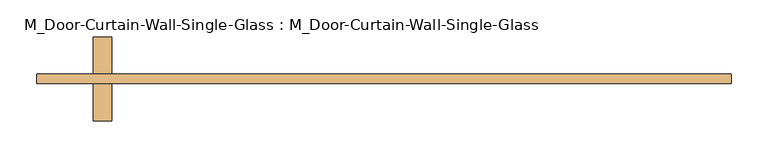
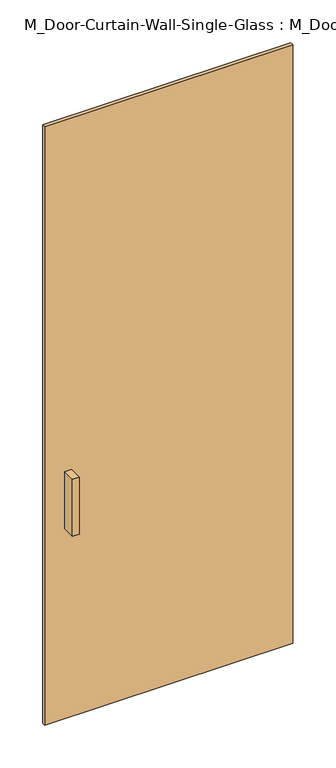
"""IFC4 building model written with IfcOpenShell, lengths in millimetres: door geometry, M_Door-Curtain-Wall-Single-Glass : M_Door-Curtain-Wall-Single-Glass."""

from ifc_helpers import new_model, si_unit, frame, origin, origin_with_axes, place, context, project, spatial, polyline, outline, extrude, source, transform, mapped, element, save


def m_door_curtain_wall_single_glass_m_door_curtain_wall_single_a386b0a2(model_context):
    return source(origin(), model_context, "Body", "SweptSolid", [
        extrude(outline(polyline([(470.8333334, 50.8), (470.8333334, 38.1), (-470.8333334, 38.1), (-470.8333334, 50.8), (470.8333334, 50.8)])), origin_with_axes(), (0.0, 0.0, 1.0), 2400.0),
        extrude(outline(polyline([(-394.6333334, 101.6), (-369.2333334, 101.6), (-369.2333334, 50.8), (-394.6333334, 50.8), (-394.6333334, 101.6)])), frame((0.0, 0.0, 762.0), z_axis=(0.0, 0.0, 1.0), x_axis=(1.0, 0.0, 0.0)), (0.0, 0.0, 1.0), 228.6),
        extrude(outline(polyline([(-369.2333334, -12.7), (-394.6333334, -12.7), (-394.6333334, 38.1), (-369.2333334, 38.1), (-369.2333334, -12.7)])), frame((0.0, 0.0, 762.0), z_axis=(0.0, 0.0, 1.0), x_axis=(1.0, 0.0, 0.0)), (0.0, 0.0, 1.0), 228.6),
    ])


if __name__ == "__main__":
    model = new_model("IFC4")
    model_context = context("Model", 3, world=origin())
    ifc_project = project(units=[si_unit("LENGTHUNIT", "METRE", prefix="MILLI")], contexts=[model_context])
    site = spatial("IfcSite", under=ifc_project)
    building = spatial("IfcBuilding", under=site)
    placement = place(None, origin())
    m_door_curtain_wall_single_glass_m_door_curtain_wall_single_shape = m_door_curtain_wall_single_glass_m_door_curtain_wall_single_a386b0a2(model_context)
    element("IfcDoor", 1, ObjectType="M_Door-Curtain-Wall-Single-Glass : M_Door-Curtain-Wall-Single-Glass", at=placement, inside=building, context=model_context, shape_type="MappedRepresentation", body=[
        mapped(m_door_curtain_wall_single_glass_m_door_curtain_wall_single_shape, transform((0.0, 0.0, 0.0), x_axis=(1.0, 0.0, 0.0), y_axis=(0.0, 1.0, 0.0), z_axis=(0.0, 0.0, 1.0))),
    ])
    save(model, "model.ifc")

# Revit data of these elements
# Type "M_Door-Curtain-Wall-Single-Glass : M_Door-Curtain-Wall-Single-Glass"
#   Type Mark = "46"
#   Assembly Code = "B2030100"
#   Analytic Construction = "<None>"
#   Width [instance default] = 900 mm
#   Thermal Resistance (R) = 1.7611 (m²·K)/W
#   Swing Angle [instance default] = 90.00°
#   Heat Transfer Coefficient (U) = 0.567826 W/(m²·K)
#   Offset = 50.8 mm
#   Define Thermal Properties by = 1
#   Function = 1
#   Door Handle Material = Aluminum
#   Glazing = Glass
#   Visual Light Transmittance = 0
#   Solar Heat Gain Coefficient = 0
#   Construction Type Id = ""
# Element 1 (IfcDoor, "M_Door-Curtain-Wall-Single-Glass : M_Door-Curtain-Wall-Single-Glass")
#   Width = 941.667 mm
#   Materials on its faces: "Aluminum", "Glass"
# Materials
#   "Aluminum": class "Metal", colour RGB 247 247 247, transparency 0, Description = "Aluminum 6061", Cost = 0
#   "Glass": class "Glass", colour RGB 0 128 192, transparency 0.9, Description = "Soda Lime Glass", Cost = 0
